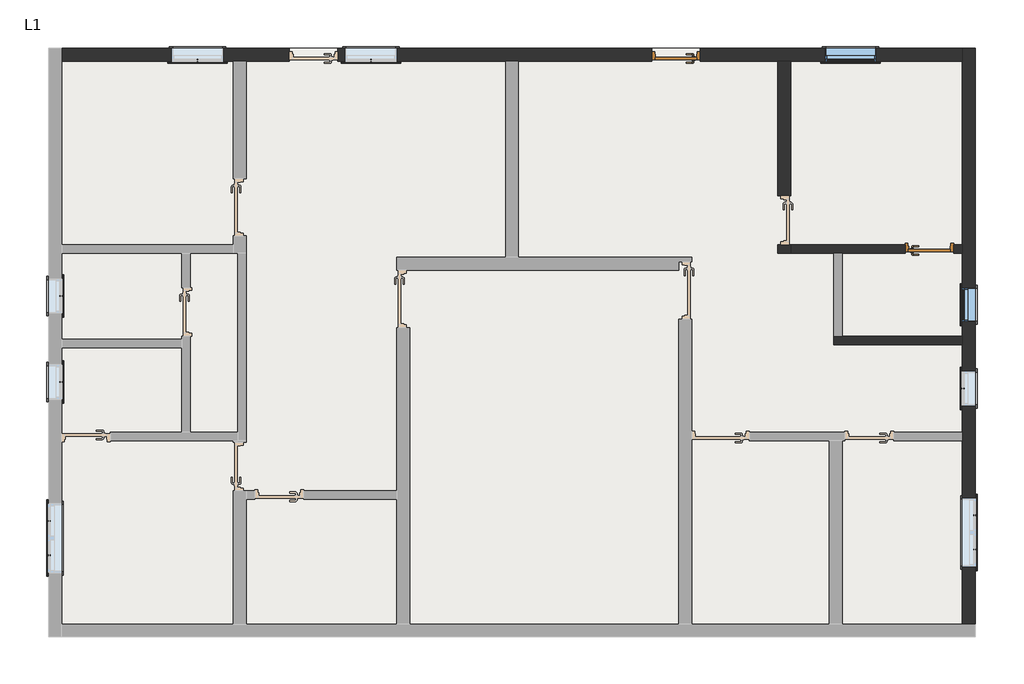
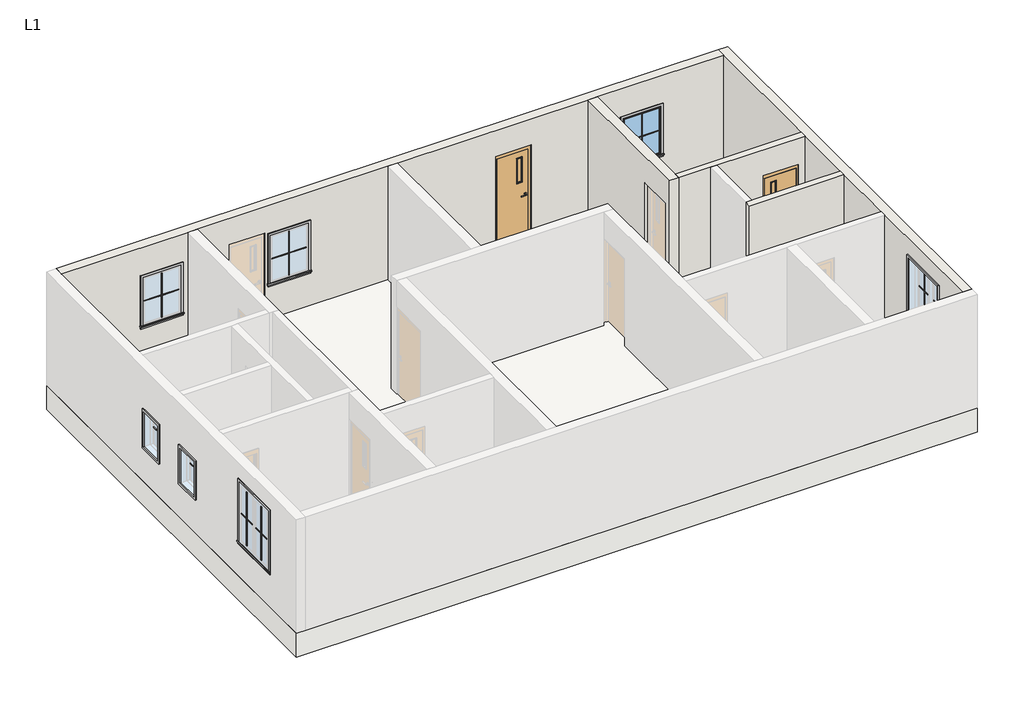
# One storey, part 2 of 2: 29 proxies, 5 walls, 2 doors, 2 windows, 1 slab.
"""IFC4 building model written with IfcOpenShell, lengths in millimetres."""

from ifc_helpers import new_model, si_unit, origin, origin_with_axes, place, context, project, spatial, polyline, outline, extrude, faceted_brep, transform, mapped, element, save
from components import muntin_pattern_2x2_muntin_pattern_2x2_0b2f62cf, muntin_pattern_2x2_muntin_pattern_2x2_f7d54b4d, muntin_pattern_2x2_muntin_pattern_2x2_6dad3731, muntin_pattern_2x2_muntin_pattern_2x2_a30a3345, trim_window_exterior_flat_with_sill_e4b28ec3, trim_window_exterior_flat_with_sill_a665a915, trim_window_exterior_flat_with_sill_92b9b949, trim_window_interior_flat_picture_frame_39ff4276, trim_window_interior_flat_picture_frame_d485c387, trim_window_interior_flat_picture_frame_3bb882cf, door_e76c17f4, door_21b9ace8, window_b8e47f08, window_2799360a

model = new_model("IFC4")

# Units and contexts
model_context = context("Model", 3, world=origin())
ifc_project = project(units=[si_unit("LENGTHUNIT", "METRE", prefix="MILLI")], contexts=[model_context])

# Site, building, storey
site = spatial("IfcSite", under=ifc_project)
building = spatial("IfcBuilding", under=site)
storey = spatial("IfcBuildingStorey", under=building, Name="L1", Elevation=609.6)

# Proxies
placement = place(None, origin())
muntin_pattern_2x2_muntin_pattern_2x2_shape = muntin_pattern_2x2_muntin_pattern_2x2_0b2f62cf(model_context)
element("IfcBuildingElementProxy", 1, Name="Muntin Pattern_2x2 : Muntin Pattern_2x2", ObjectType="Muntin Pattern_2x2 : Muntin Pattern_2x2", at=placement, inside=storey, context=model_context, shape_type="MappedRepresentation", body=[
    mapped(muntin_pattern_2x2_muntin_pattern_2x2_shape, transform((-3356.8879185, 5229.7528379, 1562.1), x_axis=(1.0, 0.0, 0.0), y_axis=(0.0, 1.0, 0.0), z_axis=(0.0, 0.0, 1.0))),
])
element("IfcBuildingElementProxy", 2, Name="Muntin Pattern_2x2 : Muntin Pattern_2x2", ObjectType="Muntin Pattern_2x2 : Muntin Pattern_2x2", at=placement, inside=storey, context=model_context, shape_type="MappedRepresentation", body=[
    mapped(muntin_pattern_2x2_muntin_pattern_2x2_shape, transform((-283.4879185, 5229.7528379, 1562.1), x_axis=(1.0, 0.0, 0.0), y_axis=(0.0, 1.0, 0.0), z_axis=(0.0, 0.0, 1.0))),
])
element("IfcBuildingElementProxy", 3, Name="Muntin Pattern_2x2 : Muntin Pattern_2x2", ObjectType="Muntin Pattern_2x2 : Muntin Pattern_2x2", at=placement, inside=storey, context=model_context, shape_type="MappedRepresentation", body=[
    mapped(muntin_pattern_2x2_muntin_pattern_2x2_shape, transform((8225.5120815, 5229.7528379, 1562.1), x_axis=(1.0, 0.0, 0.0), y_axis=(0.0, 1.0, 0.0), z_axis=(0.0, 0.0, 1.0))),
])
muntin_pattern_2x2_muntin_pattern_2x2_2_shape = muntin_pattern_2x2_muntin_pattern_2x2_f7d54b4d(model_context)
element("IfcBuildingElementProxy", 4, Name="Muntin Pattern_2x2 : Muntin Pattern_2x2", ObjectType="Muntin Pattern_2x2 : Muntin Pattern_2x2", at=placement, inside=storey, context=model_context, shape_type="MappedRepresentation", body=[
    mapped(muntin_pattern_2x2_muntin_pattern_2x2_2_shape, transform((-5779.4129185, -469.3721621, 1562.1), x_axis=(0.0, 1.0, 0.0), y_axis=(-1.0, 0.0, 0.0), z_axis=(0.0, 0.0, 1.0))),
])
element("IfcBuildingElementProxy", 5, Name="Muntin Pattern_2x2 : Muntin Pattern_2x2", ObjectType="Muntin Pattern_2x2 : Muntin Pattern_2x2", at=placement, inside=storey, context=model_context, shape_type="MappedRepresentation", body=[
    mapped(muntin_pattern_2x2_muntin_pattern_2x2_2_shape, transform((-5779.4129185, 1054.6278379, 1562.1), x_axis=(0.0, 1.0, 0.0), y_axis=(-1.0, 0.0, 0.0), z_axis=(0.0, 0.0, 1.0))),
])
element("IfcBuildingElementProxy", 6, Name="Muntin Pattern_2x2 : Muntin Pattern_2x2", ObjectType="Muntin Pattern_2x2 : Muntin Pattern_2x2", at=placement, inside=storey, context=model_context, shape_type="MappedRepresentation", body=[
    mapped(muntin_pattern_2x2_muntin_pattern_2x2_2_shape, transform((10216.2370815, 902.2278379, 1562.1), x_axis=(0.0, -1.0, 0.0), y_axis=(1.0, 0.0, 0.0), z_axis=(0.0, 0.0, 1.0))),
])
element("IfcBuildingElementProxy", 7, Name="Muntin Pattern_2x2 : Muntin Pattern_2x2", ObjectType="Muntin Pattern_2x2 : Muntin Pattern_2x2", at=placement, inside=storey, context=model_context, shape_type="MappedRepresentation", body=[
    mapped(muntin_pattern_2x2_muntin_pattern_2x2_2_shape, transform((10216.2370815, -583.6721621, 1562.1), x_axis=(0.0, -1.0, 0.0), y_axis=(1.0, 0.0, 0.0), z_axis=(0.0, 0.0, 1.0))),
])
muntin_pattern_2x2_muntin_pattern_2x2_3_shape = muntin_pattern_2x2_muntin_pattern_2x2_6dad3731(model_context)
element("IfcBuildingElementProxy", 8, Name="Muntin Pattern_2x2 : Muntin Pattern_2x2", ObjectType="Muntin Pattern_2x2 : Muntin Pattern_2x2", at=placement, inside=storey, context=model_context, shape_type="MappedRepresentation", body=[
    mapped(muntin_pattern_2x2_muntin_pattern_2x2_3_shape, transform((10425.7870815, -2833.1596621, 1593.85), x_axis=(0.0, -1.0, 0.0), y_axis=(1.0, 0.0, 0.0), z_axis=(0.0, 0.0, 1.0))),
])
element("IfcBuildingElementProxy", 9, Name="Muntin Pattern_2x2 : Muntin Pattern_2x2", ObjectType="Muntin Pattern_2x2 : Muntin Pattern_2x2", at=placement, inside=storey, context=model_context, shape_type="MappedRepresentation", body=[
    mapped(muntin_pattern_2x2_muntin_pattern_2x2_3_shape, transform((-5988.9629185, -3541.1846621, 1593.85), x_axis=(0.0, 1.0, 0.0), y_axis=(-1.0, 0.0, 0.0), z_axis=(0.0, 0.0, 1.0))),
])
muntin_pattern_2x2_muntin_pattern_2x2_4_shape = muntin_pattern_2x2_muntin_pattern_2x2_a30a3345(model_context)
element("IfcBuildingElementProxy", 10, Name="Muntin Pattern_2x2 : Muntin Pattern_2x2", ObjectType="Muntin Pattern_2x2 : Muntin Pattern_2x2", at=placement, inside=storey, context=model_context, shape_type="MappedRepresentation", body=[
    mapped(muntin_pattern_2x2_muntin_pattern_2x2_4_shape, transform((10425.7870815, -3439.5846621, 1593.85), x_axis=(0.0, 1.0, 0.0), y_axis=(-1.0, 0.0, 0.0), z_axis=(0.0, 0.0, 1.0))),
])
element("IfcBuildingElementProxy", 11, Name="Muntin Pattern_2x2 : Muntin Pattern_2x2", ObjectType="Muntin Pattern_2x2 : Muntin Pattern_2x2", at=placement, inside=storey, context=model_context, shape_type="MappedRepresentation", body=[
    mapped(muntin_pattern_2x2_muntin_pattern_2x2_4_shape, transform((-5988.9629185, -2934.7596621, 1593.85), x_axis=(0.0, -1.0, 0.0), y_axis=(1.0, 0.0, 0.0), z_axis=(0.0, 0.0, 1.0))),
])
trim_window_exterior_flat_with_sill_shape = trim_window_exterior_flat_with_sill_e4b28ec3(model_context)
element("IfcBuildingElementProxy", 12, Name="Trim-Window-Exterior-Flat : with Sill", ObjectType="Trim-Window-Exterior-Flat : with Sill", at=placement, inside=storey, context=model_context, shape_type="MappedRepresentation", body=[
    mapped(trim_window_exterior_flat_with_sill_shape, transform((-3356.8879185, 5220.2278379, 2743.2), x_axis=(1.0, 0.0, 0.0), y_axis=(0.0, 0.0, 1.0), z_axis=(0.0, -1.0, 0.0))),
])
element("IfcBuildingElementProxy", 13, Name="Trim-Window-Exterior-Flat : with Sill", ObjectType="Trim-Window-Exterior-Flat : with Sill", at=placement, inside=storey, context=model_context, shape_type="MappedRepresentation", body=[
    mapped(trim_window_exterior_flat_with_sill_shape, transform((-283.4879185, 5220.2278379, 2743.2), x_axis=(1.0, 0.0, 0.0), y_axis=(0.0, 0.0, 1.0), z_axis=(0.0, -1.0, 0.0))),
])
element("IfcBuildingElementProxy", 14, Name="Trim-Window-Exterior-Flat : with Sill", ObjectType="Trim-Window-Exterior-Flat : with Sill", at=placement, inside=storey, context=model_context, shape_type="MappedRepresentation", body=[
    mapped(trim_window_exterior_flat_with_sill_shape, transform((8225.5120815, 5220.2278379, 2743.2), x_axis=(1.0, 0.0, 0.0), y_axis=(0.0, 0.0, 1.0), z_axis=(0.0, -1.0, 0.0))),
])
trim_window_exterior_flat_with_sill_2_shape = trim_window_exterior_flat_with_sill_a665a915(model_context)
element("IfcBuildingElementProxy", 15, Name="Trim-Window-Exterior-Flat : with Sill", ObjectType="Trim-Window-Exterior-Flat : with Sill", at=placement, inside=storey, context=model_context, shape_type="MappedRepresentation", body=[
    mapped(trim_window_exterior_flat_with_sill_2_shape, transform((-5769.8879185, -469.3721621, 2438.4), x_axis=(0.0, 1.0, 0.0), y_axis=(0.0, 0.0, 1.0), z_axis=(1.0, 0.0, 0.0))),
])
element("IfcBuildingElementProxy", 16, Name="Trim-Window-Exterior-Flat : with Sill", ObjectType="Trim-Window-Exterior-Flat : with Sill", at=placement, inside=storey, context=model_context, shape_type="MappedRepresentation", body=[
    mapped(trim_window_exterior_flat_with_sill_2_shape, transform((-5769.8879185, 1054.6278379, 2438.4), x_axis=(0.0, 1.0, 0.0), y_axis=(0.0, 0.0, 1.0), z_axis=(1.0, 0.0, 0.0))),
])
element("IfcBuildingElementProxy", 17, Name="Trim-Window-Exterior-Flat : with Sill", ObjectType="Trim-Window-Exterior-Flat : with Sill", at=placement, inside=storey, context=model_context, shape_type="MappedRepresentation", body=[
    mapped(trim_window_exterior_flat_with_sill_2_shape, transform((10206.7120815, 902.2278379, 2438.4), x_axis=(0.0, -1.0, 0.0), y_axis=(0.0, 0.0, 1.0), z_axis=(-1.0, 0.0, 0.0))),
])
element("IfcBuildingElementProxy", 18, Name="Trim-Window-Exterior-Flat : with Sill", ObjectType="Trim-Window-Exterior-Flat : with Sill", at=placement, inside=storey, context=model_context, shape_type="MappedRepresentation", body=[
    mapped(trim_window_exterior_flat_with_sill_2_shape, transform((10206.7120815, -583.6721621, 2438.4), x_axis=(0.0, -1.0, 0.0), y_axis=(0.0, 0.0, 1.0), z_axis=(-1.0, 0.0, 0.0))),
])
trim_window_exterior_flat_with_sill_3_shape = trim_window_exterior_flat_with_sill_92b9b949(model_context)
element("IfcBuildingElementProxy", 19, Name="Trim-Window-Exterior-Flat : with Sill", ObjectType="Trim-Window-Exterior-Flat : with Sill", at=placement, inside=storey, context=model_context, shape_type="MappedRepresentation", body=[
    mapped(trim_window_exterior_flat_with_sill_3_shape, transform((10435.3120815, -3136.3721621, 3048.0), x_axis=(0.0, 1.0, 0.0), y_axis=(0.0, 0.0, 1.0), z_axis=(1.0, 0.0, 0.0))),
])
element("IfcBuildingElementProxy", 20, Name="Trim-Window-Exterior-Flat : with Sill", ObjectType="Trim-Window-Exterior-Flat : with Sill", at=placement, inside=storey, context=model_context, shape_type="MappedRepresentation", body=[
    mapped(trim_window_exterior_flat_with_sill_3_shape, transform((-5998.4879185, -3237.9721621, 3048.0), x_axis=(0.0, -1.0, 0.0), y_axis=(0.0, 0.0, 1.0), z_axis=(-1.0, 0.0, 0.0))),
])
trim_window_interior_flat_picture_frame_shape = trim_window_interior_flat_picture_frame_39ff4276(model_context)
element("IfcBuildingElementProxy", 21, Name="Trim-Window-Interior-Flat : Picture Frame", ObjectType="Trim-Window-Interior-Flat : Picture Frame", at=placement, inside=storey, context=model_context, shape_type="MappedRepresentation", body=[
    mapped(trim_window_interior_flat_picture_frame_shape, transform((-3356.8879185, 5448.8278379, 2743.2), x_axis=(-1.0, 0.0, 0.0), y_axis=(0.0, 0.0, 1.0), z_axis=(0.0, 1.0, 0.0))),
])
element("IfcBuildingElementProxy", 22, Name="Trim-Window-Interior-Flat : Picture Frame", ObjectType="Trim-Window-Interior-Flat : Picture Frame", at=placement, inside=storey, context=model_context, shape_type="MappedRepresentation", body=[
    mapped(trim_window_interior_flat_picture_frame_shape, transform((-283.4879185, 5448.8278379, 2743.2), x_axis=(-1.0, 0.0, 0.0), y_axis=(0.0, 0.0, 1.0), z_axis=(0.0, 1.0, 0.0))),
])
element("IfcBuildingElementProxy", 23, Name="Trim-Window-Interior-Flat : Picture Frame", ObjectType="Trim-Window-Interior-Flat : Picture Frame", at=placement, inside=storey, context=model_context, shape_type="MappedRepresentation", body=[
    mapped(trim_window_interior_flat_picture_frame_shape, transform((8225.5120815, 5448.8278379, 2743.2), x_axis=(-1.0, 0.0, 0.0), y_axis=(0.0, 0.0, 1.0), z_axis=(0.0, 1.0, 0.0))),
])
trim_window_interior_flat_picture_frame_2_shape = trim_window_interior_flat_picture_frame_d485c387(model_context)
element("IfcBuildingElementProxy", 24, Name="Trim-Window-Interior-Flat : Picture Frame", ObjectType="Trim-Window-Interior-Flat : Picture Frame", at=placement, inside=storey, context=model_context, shape_type="MappedRepresentation", body=[
    mapped(trim_window_interior_flat_picture_frame_2_shape, transform((-5998.4879185, -469.3721621, 2438.4), x_axis=(0.0, -1.0, 0.0), y_axis=(0.0, 0.0, 1.0), z_axis=(-1.0, 0.0, 0.0))),
])
element("IfcBuildingElementProxy", 25, Name="Trim-Window-Interior-Flat : Picture Frame", ObjectType="Trim-Window-Interior-Flat : Picture Frame", at=placement, inside=storey, context=model_context, shape_type="MappedRepresentation", body=[
    mapped(trim_window_interior_flat_picture_frame_2_shape, transform((-5998.4879185, 1054.6278379, 2438.4), x_axis=(0.0, -1.0, 0.0), y_axis=(0.0, 0.0, 1.0), z_axis=(-1.0, 0.0, 0.0))),
])
element("IfcBuildingElementProxy", 26, Name="Trim-Window-Interior-Flat : Picture Frame", ObjectType="Trim-Window-Interior-Flat : Picture Frame", at=placement, inside=storey, context=model_context, shape_type="MappedRepresentation", body=[
    mapped(trim_window_interior_flat_picture_frame_2_shape, transform((10435.3120815, 902.2278379, 2438.4), x_axis=(0.0, 1.0, 0.0), y_axis=(0.0, 0.0, 1.0), z_axis=(1.0, 0.0, 0.0))),
])
element("IfcBuildingElementProxy", 27, Name="Trim-Window-Interior-Flat : Picture Frame", ObjectType="Trim-Window-Interior-Flat : Picture Frame", at=placement, inside=storey, context=model_context, shape_type="MappedRepresentation", body=[
    mapped(trim_window_interior_flat_picture_frame_2_shape, transform((10435.3120815, -583.6721621, 2438.4), x_axis=(0.0, 1.0, 0.0), y_axis=(0.0, 0.0, 1.0), z_axis=(1.0, 0.0, 0.0))),
])
trim_window_interior_flat_picture_frame_3_shape = trim_window_interior_flat_picture_frame_3bb882cf(model_context)
element("IfcBuildingElementProxy", 28, Name="Trim-Window-Interior-Flat : Picture Frame", ObjectType="Trim-Window-Interior-Flat : Picture Frame", at=placement, inside=storey, context=model_context, shape_type="MappedRepresentation", body=[
    mapped(trim_window_interior_flat_picture_frame_3_shape, transform((10206.7120815, -3136.3721621, 3048.0), x_axis=(0.0, -1.0, 0.0), y_axis=(0.0, 0.0, 1.0), z_axis=(-1.0, 0.0, 0.0))),
])
element("IfcBuildingElementProxy", 29, Name="Trim-Window-Interior-Flat : Picture Frame", ObjectType="Trim-Window-Interior-Flat : Picture Frame", at=placement, inside=storey, context=model_context, shape_type="MappedRepresentation", body=[
    mapped(trim_window_interior_flat_picture_frame_3_shape, transform((-5769.8879185, -3237.9721621, 3048.0), x_axis=(0.0, 1.0, 0.0), y_axis=(0.0, 0.0, 1.0), z_axis=(1.0, 0.0, 0.0))),
])

# Doors
door_shape = door_e76c17f4(model_context)
element("IfcDoor", 30, ObjectType="Door-Passage-Single-Vision_Lite : 30\" x 84\"", at=placement, inside=storey, context=model_context, shape_type="MappedRepresentation", body=[
    mapped(door_shape, transform((5126.7120815, 5340.8778379, 609.6), x_axis=(-1.0, 0.0, 0.0), y_axis=(0.0, -1.0, 0.0), z_axis=(0.0, 0.0, 1.0))),
])
door_2_shape = door_21b9ace8(model_context)
element("IfcDoor", 31, ObjectType="Door-Passage-Single-Vision_Lite : 30\" x 84\"", at=placement, inside=storey, context=model_context, shape_type="MappedRepresentation", body=[
    mapped(door_2_shape, transform((9622.5120815, 1899.1778379, 609.6), x_axis=(1.0, 0.0, 0.0), y_axis=(0.0, 1.0, 0.0), z_axis=(0.0, 0.0, 1.0))),
])

# Slab
element("IfcSlab", 32, ObjectType="plinth 2'", at=placement, inside=storey, context=model_context, shape_type="SweptSolid", body=[
    extrude(outline(polyline([(10435.3120815, 5448.8278379), (10435.3120815, -4990.5721621), (-5998.4879185, -4990.5721621), (-5998.4879185, 5448.8278379), (10435.3120815, 5448.8278379)])), origin_with_axes(), (0.0, 0.0, 1.0), 609.6),
])

# Walls
element("IfcWall", 33, ObjectType="Generic - 6\"", at=placement, inside=storey, context=model_context, shape_type="Brep", body=[
    faceted_brep([(10206.7120815, 343.4278379, 609.6), (8073.1120815, 343.4278379, 609.6), (7920.7120815, 343.4278379, 609.6), (7920.7120815, 343.4278379, 3505.2), (8073.1120815, 343.4278379, 3505.2), (10206.7120815, 343.4278379, 3505.2), (10206.7120815, 191.0278379, 609.6), (10206.7120815, 191.0278379, 3505.2), (7920.7120815, 191.0278379, 3505.2), (7920.7120815, 191.0278379, 609.6)], [[[0, 1, 2, 3, 4, 5]], [[6, 7, 8, 9]], [[2, 1, 0, 6, 9]], [[0, 5, 7, 6]], [[3, 2, 9, 8]], [[5, 4, 3, 8, 7]]]),
])
element("IfcWall", 34, ObjectType="Generic - 6\"", at=placement, inside=storey, context=model_context, shape_type="Brep", body=[
    faceted_brep([(7158.7120815, 1816.6278379, 3505.2), (7158.7120815, 1816.6278379, 609.6), (7920.7120815, 1816.6278379, 609.6), (8073.1120815, 1816.6278379, 609.6), (9190.7120815, 1816.6278379, 609.6), (9190.7120815, 1816.6278379, 2844.8), (10054.3120815, 1816.6278379, 2844.8), (10054.3120815, 1816.6278379, 609.6), (10206.7120815, 1816.6278379, 609.6), (10206.7120815, 1816.6278379, 3505.2), (8073.1120815, 1816.6278379, 3505.2), (7920.7120815, 1816.6278379, 3505.2), (7158.7120815, 1969.0278379, 609.6), (7158.7120815, 1969.0278379, 3505.2), (10206.7120815, 1969.0278379, 3505.2), (10206.7120815, 1969.0278379, 609.6), (10054.3120815, 1969.0278379, 609.6), (10054.3120815, 1969.0278379, 2844.8), (9190.7120815, 1969.0278379, 2844.8), (9190.7120815, 1969.0278379, 609.6)], [[[0, 1, 2, 3, 4, 5, 6, 7, 8, 9, 10, 11]], [[12, 13, 14, 15, 16, 17, 18, 19]], [[1, 12, 19, 4, 3, 2]], [[15, 8, 7, 16]], [[1, 0, 13, 12]], [[9, 8, 15, 14]], [[6, 17, 16, 7]], [[17, 6, 5, 18]], [[18, 5, 4, 19]], [[0, 11, 10, 9, 14, 13]]]),
])
element("IfcWall", 35, ObjectType="Generic - 9\"", at=placement, inside=storey, context=model_context, shape_type="Brep", body=[
    faceted_brep([(10435.3120815, -4761.9721621, 609.6), (10435.3120815, 5448.8278379, 609.6), (10435.3120815, 5448.8278379, 3505.2), (10435.3120815, -4761.9721621, 3505.2), (10435.3120815, 1207.0278379, 2438.4), (10435.3120815, 1207.0278379, 1524.0), (10435.3120815, 597.4278379, 1524.0), (10435.3120815, 597.4278379, 2438.4), (10435.3120815, -278.8721621, 2438.4), (10435.3120815, -278.8721621, 1524.0), (10435.3120815, -888.4721621, 1524.0), (10435.3120815, -888.4721621, 2438.4), (10435.3120815, -3745.9721621, 1524.0), (10435.3120815, -3745.9721621, 3048.0), (10435.3120815, -2526.7721621, 3048.0), (10435.3120815, -2526.7721621, 1524.0), (10206.7120815, 5448.8278379, 609.6), (10206.7120815, 5220.2278379, 609.6), (10206.7120815, 1969.0278379, 609.6), (10206.7120815, 1816.6278379, 609.6), (10206.7120815, 343.4278379, 609.6), (10206.7120815, 191.0278379, 609.6), (10206.7120815, -1358.3721621, 609.6), (10206.7120815, -1510.7721621, 609.6), (10206.7120815, -4761.9721621, 609.6), (10206.7120815, -4761.9721621, 3505.2), (10206.7120815, -1510.7721621, 3505.2), (10206.7120815, -1358.3721621, 3505.2), (10206.7120815, 191.0278379, 3505.2), (10206.7120815, 343.4278379, 3505.2), (10206.7120815, 1816.6278379, 3505.2), (10206.7120815, 1969.0278379, 3505.2), (10206.7120815, 5220.2278379, 3505.2), (10206.7120815, 5448.8278379, 3505.2), (10206.7120815, 1207.0278379, 2438.4), (10206.7120815, 597.4278379, 2438.4), (10206.7120815, 597.4278379, 1524.0), (10206.7120815, 1207.0278379, 1524.0), (10206.7120815, -278.8721621, 2438.4), (10206.7120815, -888.4721621, 2438.4), (10206.7120815, -888.4721621, 1524.0), (10206.7120815, -278.8721621, 1524.0), (10206.7120815, -3745.9721621, 3048.0), (10206.7120815, -3745.9721621, 1524.0), (10206.7120815, -2526.7721621, 1524.0), (10206.7120815, -2526.7721621, 3048.0)], [[[0, 1, 2, 3], [4, 5, 6, 7], [8, 9, 10, 11], [12, 13, 14, 15]], [[16, 17, 18, 19, 20, 21, 22, 23, 24, 25, 26, 27, 28, 29, 30, 31, 32, 33], [34, 35, 36, 37], [38, 39, 40, 41], [42, 43, 44, 45]], [[1, 0, 24, 23, 22, 21, 20, 19, 18, 17, 16]], [[0, 3, 25, 24]], [[2, 1, 16, 33]], [[5, 4, 34, 37]], [[6, 5, 37, 36]], [[7, 6, 36, 35]], [[4, 7, 35, 34]], [[9, 8, 38, 41]], [[10, 9, 41, 40]], [[11, 10, 40, 39]], [[8, 11, 39, 38]], [[3, 2, 33, 32, 31, 30, 29, 28, 27, 26, 25]], [[42, 13, 12, 43]], [[43, 12, 15, 44]], [[44, 15, 14, 45]], [[13, 42, 45, 14]]]),
])
element("IfcWall", 36, ObjectType="Generic - 9\"", at=placement, inside=storey, context=model_context, shape_type="Brep", body=[
    faceted_brep([(10206.7120815, 5448.8278379, 3505.2), (10206.7120815, 5448.8278379, 609.6), (5558.5120815, 5448.8278379, 609.6), (5558.5120815, 5448.8278379, 2844.8), (4694.9120815, 5448.8278379, 2844.8), (4694.9120815, 5448.8278379, 609.6), (-867.6879185, 5448.8278379, 609.6), (-867.6879185, 5448.8278379, 2844.8), (-1731.2879185, 5448.8278379, 2844.8), (-1731.2879185, 5448.8278379, 609.6), (-5769.8879185, 5448.8278379, 609.6), (-5769.8879185, 5448.8278379, 3505.2), (-3814.0879185, 5448.8278379, 2743.2), (-3814.0879185, 5448.8278379, 1524.0), (-2899.6879185, 5448.8278379, 1524.0), (-2899.6879185, 5448.8278379, 2743.2), (-740.6879185, 5448.8278379, 2743.2), (-740.6879185, 5448.8278379, 1524.0), (173.7120815, 5448.8278379, 1524.0), (173.7120815, 5448.8278379, 2743.2), (7768.3120815, 5448.8278379, 2743.2), (7768.3120815, 5448.8278379, 1524.0), (8682.7120815, 5448.8278379, 1524.0), (8682.7120815, 5448.8278379, 2743.2), (10206.7120815, 5220.2278379, 609.6), (10206.7120815, 5220.2278379, 3505.2), (7158.7120815, 5220.2278379, 3505.2), (6930.1120815, 5220.2278379, 3505.2), (2332.7120815, 5220.2278379, 3505.2), (2104.1120815, 5220.2278379, 3505.2), (-2493.2879185, 5220.2278379, 3505.2), (-2721.8879185, 5220.2278379, 3505.2), (-5769.8879185, 5220.2278379, 3505.2), (-5769.8879185, 5220.2278379, 609.6), (-2721.8879185, 5220.2278379, 609.6), (-2493.2879185, 5220.2278379, 609.6), (-1731.2879185, 5220.2278379, 609.6), (-1731.2879185, 5220.2278379, 2844.8), (-867.6879185, 5220.2278379, 2844.8), (-867.6879185, 5220.2278379, 609.6), (2104.1120815, 5220.2278379, 609.6), (2332.7120815, 5220.2278379, 609.6), (4694.9120815, 5220.2278379, 609.6), (4694.9120815, 5220.2278379, 2844.8), (5558.5120815, 5220.2278379, 2844.8), (5558.5120815, 5220.2278379, 609.6), (6930.1120815, 5220.2278379, 609.6), (7158.7120815, 5220.2278379, 609.6), (-3814.0879185, 5220.2278379, 2743.2), (-2899.6879185, 5220.2278379, 2743.2), (-2899.6879185, 5220.2278379, 1524.0), (-3814.0879185, 5220.2278379, 1524.0), (-740.6879185, 5220.2278379, 2743.2), (173.7120815, 5220.2278379, 2743.2), (173.7120815, 5220.2278379, 1524.0), (-740.6879185, 5220.2278379, 1524.0), (7768.3120815, 5220.2278379, 2743.2), (8682.7120815, 5220.2278379, 2743.2), (8682.7120815, 5220.2278379, 1524.0), (7768.3120815, 5220.2278379, 1524.0)], [[[0, 1, 2, 3, 4, 5, 6, 7, 8, 9, 10, 11], [12, 13, 14, 15], [16, 17, 18, 19], [20, 21, 22, 23]], [[24, 25, 26, 27, 28, 29, 30, 31, 32, 33, 34, 35, 36, 37, 38, 39, 40, 41, 42, 43, 44, 45, 46, 47], [48, 49, 50, 51], [52, 53, 54, 55], [56, 57, 58, 59]], [[1, 24, 47, 46, 45, 2]], [[33, 10, 9, 36, 35, 34]], [[39, 6, 5, 42, 41, 40]], [[1, 0, 25, 24]], [[11, 10, 33, 32]], [[8, 37, 36, 9]], [[7, 38, 37, 8]], [[38, 7, 6, 39]], [[4, 43, 42, 5]], [[43, 4, 3, 44]], [[44, 3, 2, 45]], [[13, 12, 48, 51]], [[14, 13, 51, 50]], [[15, 14, 50, 49]], [[12, 15, 49, 48]], [[17, 16, 52, 55]], [[18, 17, 55, 54]], [[19, 18, 54, 53]], [[16, 19, 53, 52]], [[21, 20, 56, 59]], [[22, 21, 59, 58]], [[23, 22, 58, 57]], [[20, 23, 57, 56]], [[0, 11, 32, 31, 30, 29, 28, 27, 26, 25]]]),
])
element("IfcWall", 37, ObjectType="Generic - 9\"", at=placement, inside=storey, context=model_context, shape_type="Brep", body=[
    faceted_brep([(6930.1120815, 5220.2278379, 3505.2), (6930.1120815, 5220.2278379, 609.6), (6930.1120815, 2832.6278379, 609.6), (6930.1120815, 2832.6278379, 2844.8), (6930.1120815, 1969.0278379, 2844.8), (6930.1120815, 1969.0278379, 609.6), (6930.1120815, 1816.6278379, 609.6), (6930.1120815, 1816.6278379, 3505.2), (7158.7120815, 5220.2278379, 609.6), (7158.7120815, 5220.2278379, 3505.2), (7158.7120815, 1969.0278379, 3505.2), (7158.7120815, 1816.6278379, 3505.2), (7158.7120815, 1816.6278379, 609.6), (7158.7120815, 1969.0278379, 609.6), (7158.7120815, 1969.0278379, 2844.8), (7158.7120815, 2832.6278379, 2844.8), (7158.7120815, 2832.6278379, 609.6)], [[[0, 1, 2, 3, 4, 5, 6, 7]], [[8, 9, 10, 11, 12, 13, 14, 15, 16]], [[1, 8, 16, 2]], [[12, 6, 5, 13]], [[1, 0, 9, 8]], [[7, 6, 12, 11]], [[4, 14, 13, 5]], [[14, 4, 3, 15]], [[15, 3, 2, 16]], [[0, 7, 11, 10, 9]]]),
])

# Windows
window_shape = window_b8e47f08(model_context)
element("IfcWindow", 38, ObjectType="Window-Fixed : 24\" x 36\"", at=placement, inside=storey, context=model_context, shape_type="MappedRepresentation", body=[
    mapped(window_shape, transform((10321.0120815, 902.2278379, 609.6), x_axis=(0.0, 1.0, 0.0), y_axis=(-1.0, 0.0, 0.0), z_axis=(0.0, 0.0, 1.0))),
])
window_2_shape = window_2799360a(model_context)
element("IfcWindow", 39, ObjectType="Window-Fixed : 36\" x 48\"", at=placement, inside=storey, context=model_context, shape_type="MappedRepresentation", body=[
    mapped(window_2_shape, transform((8225.5120815, 5334.5278379, 609.6), x_axis=(-1.0, 0.0, 0.0), y_axis=(0.0, -1.0, 0.0), z_axis=(0.0, 0.0, 1.0))),
])

save(model, "model.ifc")

# Revit data of these elements
# Type "Muntin Pattern_2x2 : Muntin Pattern_2x2"
#   Width [instance default] = 4' - 0"
#   Thickness = 0' - 0 1/2"
#   Height [instance default] = 4' - 0"
#   Distance = 0' - 0 3/4"
#   Interior Material [instance default] = none
#   Exterior Material [instance default] = none
#   Default Elevation = 0
# Type "Trim-Window-Exterior-Flat : with Sill"
#   Trim Width = 0' - 2 1/4"
#   Trim Thickness_Picture Frame = 0' - 1 1/4"
#   Trim Thickness_with Sill = 0' - 0 3/4"
#   Sill Thickness = 0' - 1 1/4"
#   Opening Width [instance default] = 2' - 0"
#   Opening Height [instance default] = 3' - 0"
#   Default Elevation = 4' - 0"
#   Sill = yes
#   Picture Frame = no
#   Trim Material [instance default] = none
# Type "Trim-Window-Interior-Flat : Picture Frame"
#   Trim Thickness_Picture Frame = 0' - 1 1/4"
#   Trim Width = 0' - 2 1/4"
#   Trim Thickness_with Sill = 0' - 0 3/4"
#   Sill Thickness = 0' - 1 1/4"
#   Opening Width [instance default] = 2' - 0"
#   Opening Height [instance default] = 3' - 0"
#   Default Elevation = 4' - 0"
#   Sill = no
#   Picture Frame = yes
#   Trim Material [instance default] = none
# Type "Door-Passage-Single-Vision_Lite : 30\" x 84\""
#   Type Mark = "20"
#   Assembly Code = "B2030100"
#   Analytic Construction = "Wooden"
#   Thickness = 0' - 1 3/4"
#   Thermal Resistance (R) = 2.5876 (h·ft²·°F)/BTU
#   Swing Angle [instance default] = 90.00°
#   Strike Height = 3' - 4"
#   Rough Width [instance default] = 2' - 10"
#   Rough Height [instance default] = 7' - 4"
#   MFOpeningHeight [instance default] = 0' - 4"
#   MFOpeningWidth [instance default] = 0' - 4"
#   Inset Calculate [instance default] = 0' - 4"
#   Masonry Inset [instance default] = 0' - 1"
#   Height = 7' - 0"
#   Width = 2' - 6"
#   Heat Transfer Coefficient (U) = 0.3865 BTU/(h·ft²·°F)
#   Masonry Frame Depth = 0' - 5 3/4"
#   Masonry Frame [instance default] = yes
#   Function = 1
#   Dry Wall Frame [instance default] = no
#   Define Thermal Properties by = 1
#   Panel Material = Wood - Birch
#   Glazing = Glass
#   Glass Stop Material = Metal - Paint Finish - Grey
#   Frame Material = Metal - Paint Finish - Grey
#   Door Handle Material = Aluminum
#   Visual Light Transmittance = 0
#   Solar Heat Gain Coefficient = 0
#   Wall Closure = (empty or 0)
# Type "plinth 2'"
#   Description = "Generic Floor (Material By Category), 12\" thick"
#   Assembly Code = "B1010"
#   Type Mark = "G01"
#   Function = 0
#   Layers, outside or top first: 2' - 0" no material (function 1)
# Type "Generic - 6\""
#   Description = "Generic Wall (Material By Category), 6\" thick"
#   Assembly Code = "B2010"
#   Type Mark = "G04"
#   Layers, outside or top first: 0' - 6" no material (function 1)
# Type "Generic - 9\""
#   Description = "Generic Wall (Material By Category), 8\" thick"
#   Assembly Code = "B2010"
#   Type Mark = "G06"
#   Layers, outside or top first: 0' - 9" no material (function 1)
# Type "Window-Fixed : 24\" x 36\""
#   Type Mark = "18"
#   Fire Rating = "0.5h"
#   Assembly Code = "B2020100"
#   Analytic Construction = "Double glazing - domestic"
#   Window Inset [instance default] = 0' - 0"
#   Wall Thickness [instance default] = 0' - 6"
#   Visual Light Transmittance = 0.81
#   Thermal Resistance (R) = 1.8146 (h·ft²·°F)/BTU
#   Solar Heat Gain Coefficient = 0.76
#   Rough Width = 2' - 0 1/2"
#   Rough Height = 3' - 0 1/2"
#   Interior Wall Closure [instance default] = 0' - 2 1/4"
#   Height = 3' - 0"
#   Heat Transfer Coefficient (U) = 0.5511 BTU/(h·ft²·°F)
#   Frame Extension [instance default] = 0' - 0 1/4"
#   Exterior Wall Closure [instance default] = 0' - 1 1/4"
#   Extension Jamb [instance default] = 0' - 2 1/4"
#   Default Sill Height = 3' - 0"
#   Width = 2' - 0"
#   Muntin Visibility = yes
#   Interior Trim Visibility [instance default] = yes
#   Exterior Trim Visibility [instance default] = yes
#   Extension Jamb Visibility [instance default] = yes
#   Define Thermal Properties by = 1
#   Muntin Pattern = Muntin Pattern_2x2 : Muntin Pattern_2x2
#   Interior Trim Material = Wood - Stained
#   Interior Trim = Trim-Window-Interior-Flat : Picture Frame
#   Interior Frame Material = Wood - Stained
#   Glass Panel Material = Glass
#   Exterior Trim Material = Clad - White
#   Exterior Trim = Trim-Window-Exterior-Flat : with Sill
#   Exterior Frame Material = Clad - White
#   Wall Closure = (empty or 0)
# Type "Window-Fixed : 36\" x 48\""
#   Type Mark = "22"
#   Fire Rating = "0.5h"
#   Assembly Code = "B2020100"
#   Analytic Construction = "Double glazing - domestic"
#   Window Inset [instance default] = 0' - 0"
#   Wall Thickness [instance default] = 0' - 6"
#   Visual Light Transmittance = 0.81
#   Thermal Resistance (R) = 1.8146 (h·ft²·°F)/BTU
#   Solar Heat Gain Coefficient = 0.76
#   Rough Width = 3' - 0 1/2"
#   Rough Height = 4' - 0 1/2"
#   Interior Wall Closure [instance default] = 0' - 2 1/4"
#   Height = 4' - 0"
#   Heat Transfer Coefficient (U) = 0.5511 BTU/(h·ft²·°F)
#   Frame Extension [instance default] = 0' - 0 1/4"
#   Exterior Wall Closure [instance default] = 0' - 1 1/4"
#   Extension Jamb [instance default] = 0' - 2 1/4"
#   Default Sill Height = 3' - 0"
#   Width = 3' - 0"
#   Muntin Visibility = yes
#   Interior Trim Visibility [instance default] = yes
#   Exterior Trim Visibility [instance default] = yes
#   Extension Jamb Visibility [instance default] = yes
#   Define Thermal Properties by = 1
#   Muntin Pattern = Muntin Pattern_2x2 : Muntin Pattern_2x2
#   Interior Trim Material = Wood - Stained
#   Interior Trim = Trim-Window-Interior-Flat : Picture Frame
#   Interior Frame Material = Wood - Stained
#   Glass Panel Material = Glass
#   Exterior Trim Material = Clad - White
#   Exterior Trim = Trim-Window-Exterior-Flat : with Sill
#   Exterior Frame Material = Clad - White
#   Wall Closure = (empty or 0)
# Elements 1, 2, 3 (IfcBuildingElementProxy, "Muntin Pattern_2x2 : Muntin Pattern_2x2")
#   Width = 2' - 9"
#   Height = 3' - 9"
#   Interior Material = Wood - Stained
#   Exterior Material = Clad - White
#   Phase Created = New Construction
#   Materials on its faces: "Clad - White", "Wood - Stained"
# Elements 4, 5, 6, 7 (IfcBuildingElementProxy, "Muntin Pattern_2x2 : Muntin Pattern_2x2")
#   Width = 1' - 9"
#   Height = 2' - 9"
#   Interior Material = Wood - Stained
#   Exterior Material = Clad - White
#   Phase Created = New Construction
#   Materials on its faces: "Clad - White", "Wood - Stained"
# Elements 8, 9, 10, 11 (IfcBuildingElementProxy, "Muntin Pattern_2x2 : Muntin Pattern_2x2")
#   Width = 1' - 6 5/8"
#   Height = 4' - 6 1/2"
#   Interior Material = Wood - Stained
#   Exterior Material = Clad - White
#   Phase Created = New Construction
#   Materials on its faces: "Clad - White", "Wood - Stained"
# Elements 12, 13, 14 (IfcBuildingElementProxy, "Trim-Window-Exterior-Flat : with Sill")
#   Opening Width = 3' - 0"
#   Opening Height = 4' - 0"
#   Trim Material = Clad - White
#   Phase Created = New Construction
#   Materials on its faces: "Clad - White"
# Elements 15, 16, 17, 18 (IfcBuildingElementProxy, "Trim-Window-Exterior-Flat : with Sill")
#   Opening Width = 2' - 0"
#   Opening Height = 3' - 0"
#   Trim Material = Clad - White
#   Phase Created = New Construction
#   Materials on its faces: "Clad - White"
# Elements 19, 20 (IfcBuildingElementProxy, "Trim-Window-Exterior-Flat : with Sill")
#   Opening Width = 4' - 0"
#   Opening Height = 5' - 0"
#   Trim Material = Clad - White
#   Phase Created = New Construction
#   Materials on its faces: "Clad - White"
# Elements 21, 22, 23 (IfcBuildingElementProxy, "Trim-Window-Interior-Flat : Picture Frame")
#   Opening Width = 3' - 0"
#   Opening Height = 4' - 0"
#   Trim Material = Wood - Stained
#   Phase Created = New Construction
#   Materials on its faces: "Wood - Stained"
# Elements 24, 25, 26, 27 (IfcBuildingElementProxy, "Trim-Window-Interior-Flat : Picture Frame")
#   Opening Width = 2' - 0"
#   Opening Height = 3' - 0"
#   Trim Material = Wood - Stained
#   Phase Created = New Construction
#   Materials on its faces: "Wood - Stained"
# Elements 28, 29 (IfcBuildingElementProxy, "Trim-Window-Interior-Flat : Picture Frame")
#   Opening Width = 4' - 0"
#   Opening Height = 5' - 0"
#   Trim Material = Wood - Stained
#   Phase Created = New Construction
#   Materials on its faces: "Wood - Stained"
# Elements 30, 31 (IfcDoor, "Door-Passage-Single-Vision_Lite : 30\" x 84\"")
#   Swing Angle = 90.00°
#   Rough Width = 2' - 10"
#   Rough Height = 7' - 4"
#   Masonry Inset = 0' - 1"
#   MFOpeningWidth = 0' - 4"
#   MFOpeningHeight = 0' - 4"
#   Inset Calculate = 0' - 4"
#   Masonry Frame = yes
#   Dry Wall Frame = no
#   Phase Created = New Construction
#   Materials on its faces: "Metal - Paint Finish - Grey", "Aluminum", "Wood - Birch", "Glass"
# Element 32 (IfcSlab, "plinth 2'")
#   Height Offset From Level = 0' - 0"
#   Phase Created = New Construction
#   Materials on its faces: "Default Floor"
# Elements 33, 34 (IfcWall, "Generic - 6\"")
#   Top Offset = 0' - 0"
#   Base Offset = 0' - 0"
#   wall height = 9' - 6"
#   Phase Created = New Construction
#   Base Constraint = L1
#   Top Constraint = L2
#   Materials on its faces: "Default Wall"
# Elements 35, 36, 37 (IfcWall, "Generic - 9\"")
#   Top Offset = 0' - 0"
#   Base Offset = 0' - 0"
#   wall height = 9' - 6"
#   Phase Created = New Construction
#   Base Constraint = L1
#   Top Constraint = L2
#   Materials on its faces: "Default Wall"
# Element 38 (IfcWindow, "Window-Fixed : 24\" x 36\"")
#   Mark = "105"
#   Window Inset = 0' - 0"
#   Interior Wall Closure = 0' - 2 1/4"
#   Frame Extension = 0' - 0 1/4"
#   Exterior Wall Closure = 0' - 1 1/4"
#   Interior Trim Visibility = yes
#   Exterior Trim Visibility = yes
#   Phase Created = New Construction
#   Materials on its faces: "Wood - Stained", "Glass", "Clad - White"
# Element 39 (IfcWindow, "Window-Fixed : 36\" x 48\"")
#   Mark = "102"
#   Window Inset = 0' - 0"
#   Interior Wall Closure = 0' - 2 1/4"
#   Frame Extension = 0' - 0 1/4"
#   Exterior Wall Closure = 0' - 1 1/4"
#   Interior Trim Visibility = yes
#   Exterior Trim Visibility = yes
#   Phase Created = New Construction
#   Materials on its faces: "Wood - Stained", "Glass", "Clad - White"
# Materials
#   "Wood - Birch": class "Wood", colour RGB 173 132 96, transparency 0, Cost = 0
#   "Glass": class "Glass", colour RGB 245 245 243, transparency 1, Description = "Soda Lime Glass", Cost = 0
#   "Metal - Paint Finish - Grey": class "Paint", colour RGB 178 178 178, transparency 0, Cost = 0
#   "Aluminum": class "Metal", colour RGB 244 245 246, transparency 0, Description = "Aluminum 6061", Cost = 0
#   "Wood - Stained": class "Wood", colour RGB 173 132 96, transparency 0, Cost = 0
#   "Clad - White": class "Wood", colour RGB 245 245 243, transparency 0, Cost = 0
#   "Default Floor": colour RGB 128 128 128, transparency 0, Cost = 0
#   "Default Wall": colour RGB 192 192 192, transparency 0, Cost = 0
